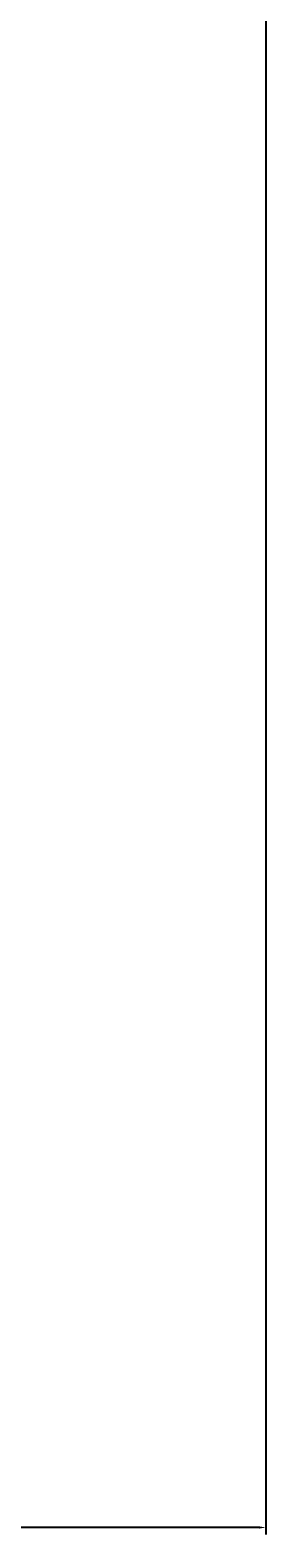
# Model space of a CAD drawing. Units: inches. Extents: x -173 to 545, y -746 to 104.
# Tile 9 of 32: x 300 to 306, y -741 to -702. Entities that reach past the tile are written whole.
import ezdxf

# ---------------------------------------------------------------- set-up
doc = ezdxf.new("R2010")
doc.units = ezdxf.units.IN
doc.header["$MEASUREMENT"] = 0
doc.layers.add('A-ANNO-DIMS', color=2, linetype='Continuous', lineweight=18)
doc.styles.get("Standard").update_dxf_attribs({"font": 'arial.ttf'})
doc.dimstyles.get("Standard").update_dxf_attribs({"dimtxt": 0.18, "dimasz": 0.18, "dimexe": 0.18, "dimexo": 0.0625, "dimgap": 0.09, "dimtad": 0, "dimtih": 1, "dimtoh": 1, "dimdec": 0, "dimzin": 0, "dimdsep": 46, "dimlunit": 3, "dimtxsty": 'Standard', "dimcen": 0.09, "dimadec": 0, "dimazin": 0, "dimtfac": 1, "dimtdec": 0, "dimtofl": 0, "dimtmove": 0, "dimatfit": 3, "dimfxl": 1, "dimtolj": 1, "dimtzin": 0, "dimarcsym": 0})

# ---------------------------------------------------------------- blocks, each defined once
blk = doc.blocks.new('*D81')
at = {"layer": 'A-ANNO-DIMS', "color": 0, "lineweight": -2, "transparency": 16777216}
for p, q in [((219.801, -551.924), (219.801, -740.642)), ((306.301, -551.924), (306.301, -740.642)), ((219.981, -740.462), (262.513, -740.462)), ((306.121, -740.462), (263.59, -740.462))]:
    blk.add_line(p, q, dxfattribs=at)
at = {"layer": 'A-ANNO-DIMS', "color": 0, "transparency": 16777216}
for points in [[(219.981, -740.432), (219.981, -740.492), (219.801, -740.462)], [(306.121, -740.432), (306.121, -740.492), (306.301, -740.462)]]:
    blk.add_solid(points, dxfattribs=at)
at = {"layer": 'Defpoints', "color": 0, "transparency": 16777216}
for p in [(219.801, -551.862), (306.301, -551.862), (306.301, -740.462)]:
    blk.add_point(p, dxfattribs=at)
at = {"layer": 'A-ANNO-DIMS', "color": 0, "transparency": 16777216, "insert": (263.051, -740.462), "char_height": 0.18, "attachment_point": 5}
blk.add_mtext('\\A1;7\'-2 1/2"', dxfattribs=at)

msp = doc.modelspace()

# ---------------------------------------------------------------- dimensions: what is measured, and where the dimension line sits
at = {"layer": 'A-ANNO-DIMS'}
dim = msp.add_linear_dim(base=(306.301, -740.462), p1=(219.801, -551.862), p2=(306.301, -551.862), dimstyle='Standard', override={"dimdec": 1, "dimlfac": 1, "dimrnd": 0, "dimzin": 1, "dimdsep": 46, "dimlunit": 4, "dimfrac": 2}, dxfattribs=at)
dim.commit()
dim.dimension.update_dxf_attribs({"geometry": '*D81', "text_midpoint": (263.051, -740.462)})

doc.saveas('drawing.dxf')
